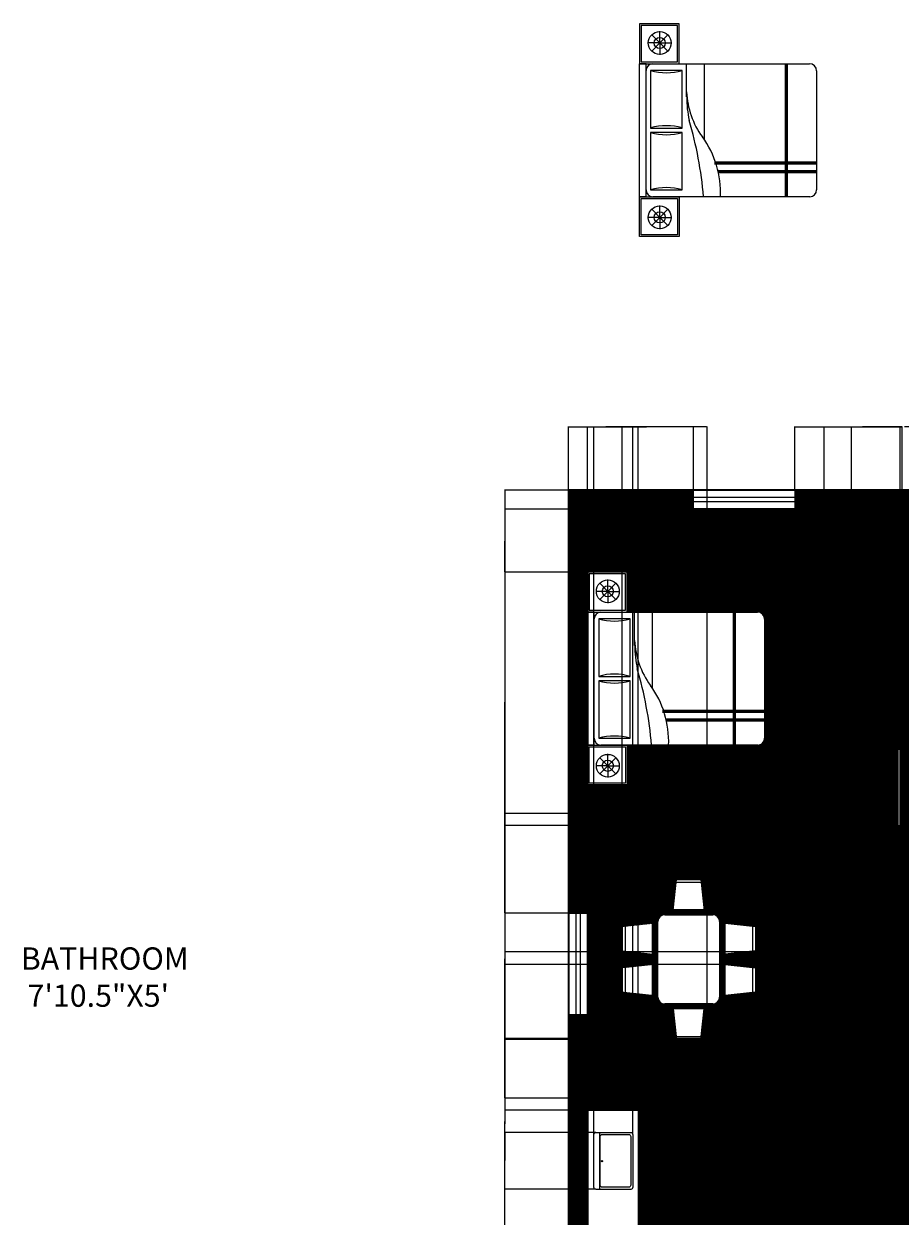
# Model space of a CAD drawing. Units: inches. Extents: x 205 to 1667, y -23 to 828.
# Tile 6 of 10: x 205 to 619, y 264 to 828. Entities that reach past the tile are written whole.
import ezdxf

# ---------------------------------------------------------------- set-up
doc = ezdxf.new("R2010")
doc.units = ezdxf.units.IN
doc.header["$MEASUREMENT"] = 0
for name, color, linetype, lineweight in [('A-ANNO-DIMS', 2, 'Continuous', 18), ('A-AREA-IDEN', 7, 'Continuous', 25), ('A-DOOR', 4, 'Continuous', 25), ('A-FLOR-CASE', 32, 'Continuous', 25), ('A-FLOR-FIXT', 9, 'Continuous', 18), ('A-FURN', 8, 'Continuous', 18), ('A-GLAZ', 4, 'Continuous', 18), ('A-WALL', 7, 'Continuous', 35)]:
    doc.layers.add(name, color=color, linetype=linetype, lineweight=lineweight)
doc.layers.add('A-FLOR-PATT', color=9, linetype='Continuous', lineweight=9, true_color=0xc7c8ca)
doc.styles.get("Standard").update_dxf_attribs({"font": 'arial.ttf'})
doc.dimstyles.get("Standard").update_dxf_attribs({"dimtxt": 0.18, "dimasz": 0.18, "dimexe": 0.18, "dimexo": 0.0625, "dimgap": 0.09, "dimtad": 0, "dimtih": 1, "dimtoh": 1, "dimdec": 4, "dimzin": 0, "dimdsep": 46, "dimtxsty": 'Standard', "dimcen": 0.09, "dimadec": 0, "dimazin": 0, "dimtfac": 1, "dimtdec": 4, "dimtofl": 0, "dimtmove": 0, "dimatfit": 3, "dimfxl": 1, "dimtolj": 1, "dimtzin": 0, "dimarcsym": 0})

# ---------------------------------------------------------------- blocks, each defined once
blk = doc.blocks.new('A$C068671E6')
for p, q in [((0, 1.55), (0, 2)), ((0, 2), (0.45, 2)), ((0.02, 1.57), (0.02, 1.98)), ((0.02, 1.98), (0.43, 1.98)), ((0.216, 1.77), (0.216, 1.905)), ((0.43, 1.98), (0.43, 1.57)), ((0.45, 2), (0.45, 1.55)), ((1.951, 2), (1.951, 1.55)), ((2.401, 2), (1.951, 2)), ((1.971, 1.98), (1.971, 1.57)), ((2.381, 1.98), (1.971, 1.98)), ((2.185, 1.77), (2.185, 1.905)), ((2.381, 1.57), (2.381, 1.98)), ((2.401, 1.55), (2.401, 2)), ((0.216, 1.77), (0.082, 1.77)), ((0.216, 1.77), (0.121, 1.865)), ((0.216, 1.77), (0.121, 1.675)), ((0.216, 1.77), (0.311, 1.865)), ((0.216, 1.77), (0.216, 1.636)), ((0.216, 1.77), (0.311, 1.675)), ((0.216, 1.77), (0.35, 1.77)), ((2.185, 1.77), (2.05, 1.77)), ((2.185, 1.77), (2.09, 1.865)), ((2.185, 1.77), (2.09, 1.675)), ((2.185, 1.77), (2.28, 1.865)), ((2.185, 1.77), (2.185, 1.636)), ((2.185, 1.77), (2.319, 1.77)), ((2.185, 1.77), (2.28, 1.675)), ((0.45, 1.55), (0, 1.55)), ((0.43, 1.57), (0.02, 1.57)), ((1.951, 1.55), (2.401, 1.55)), ((1.971, 1.57), (2.381, 1.57)), ((0.722, 1.115), (0.722, 0)), ((0.734, 1.115), (0.734, 0)), ((0.746, 1.115), (0.746, 0)), ((0.82, 1.151), (0.82, 0)), ((0.832, 1.151), (0.832, 0)), ((0.844, 1.151), (0.844, 0)), ((0.46, 0.352), (1.944, 0.352)), ((0.46, 0.34), (1.944, 0.34)), ((0.46, 0.328), (1.944, 0.328))]:
    blk.add_line(p, q)
at = {"linetype": 'ByBlock'}
for p, q in [((0.45, 1.924), (0.45, 2)), ((0.45, 2), (1.951, 2)), ((0.45, 1.924), (1.951, 1.924)), ((1.951, 1.924), (1.951, 2)), ((0.45, 0.076), (0.45, 1.848)), ((1.174, 1.873), (0.526, 1.873)), ((0.526, 1.873), (0.526, 1.518)), ((1.174, 1.518), (1.174, 1.873)), ((1.874, 1.873), (1.225, 1.873)), ((1.225, 1.873), (1.225, 1.518)), ((1.874, 1.518), (1.874, 1.873)), ((1.951, 1.848), (1.951, 0.08)), ((0.526, 1.518), (1.174, 1.518)), ((1.225, 1.518), (1.874, 1.518)), ((1.575, 1.467), (1.951, 1.467)), ((1.098, 1.264), (1.951, 1.264)), ((1.871, 0), (0.526, 0))]:
    blk.add_line(p, q, dxfattribs=at)
for centre, radius in [((0.216, 1.77), 0.129), ((2.185, 1.77), 0.129), ((0.216, 1.77), 0.0628), ((2.185, 1.77), 0.0628)]:
    blk.add_circle(centre, radius)
for centre, radius, start, end in [((0.526, 1.848), 0.0762, 90, 180), ((1.874, 1.848), 0.0762, 0, 90), ((-0.083, 1.695), 0.635, 343.7398, 16.2602), ((1.784, 1.695), 0.635, 163.7398, 196.2602), ((0.616, 1.695), 0.635, 343.7398, 16.2602), ((2.484, 1.695), 0.635, 163.7398, 196.2602), ((0.069, 5.66), 4.401, 274.9624, 286.3911), ((1.673, 0.534), 0.934, 92.5398, 126.0403), ((1.574, 0.247), 1.219, 89.9814, 102.4667), ((0.493, 2.153), 1.07, 267.6917, 306.1059), ((0.526, 0.076), 0.0762, 180, 270), ((1.871, 0.08), 0.08, 270, 0)]:
    blk.add_arc(centre, radius, start, end, dxfattribs=at)
blk = doc.blocks.new('A$C6D1B16CF')
for p, q in [((0.641, 1.5), (0.689, 1.943)), ((0.689, 1.943), (1.043, 1.943)), ((1.043, 1.943), (1.091, 1.5)), ((1.241, 1.5), (1.289, 1.943)), ((1.289, 1.943), (1.643, 1.943)), ((1.643, 1.943), (1.691, 1.5)), ((0.684, 1.9), (1.048, 1.9)), ((1.284, 1.9), (1.648, 1.9)), ((0.616, 1.421), (1.716, 1.421)), ((1.091, 1.5), (0.641, 1.5)), ((1.691, 1.5), (1.241, 1.5)), ((0.516, 0.621), (0.516, 1.321)), ((1.816, 1.321), (1.816, 0.621)), ((0, 1.146), (0.443, 1.194)), ((0, 0.792), (0, 1.146)), ((0.043, 0.787), (0.043, 1.151)), ((0.443, 1.194), (0.443, 0.744)), ((2.332, 1.146), (1.889, 1.194)), ((1.889, 1.194), (1.889, 0.744)), ((2.289, 0.787), (2.289, 1.151)), ((2.332, 0.792), (2.332, 1.146)), ((0.443, 0.744), (0, 0.792)), ((1.889, 0.744), (2.332, 0.792)), ((1.716, 0.521), (0.616, 0.521)), ((1.091, 0.443), (0.641, 0.443)), ((0.641, 0.443), (0.689, 0)), ((1.043, 0), (1.091, 0.443)), ((1.691, 0.443), (1.241, 0.443)), ((1.241, 0.443), (1.289, 0)), ((1.643, 0), (1.691, 0.443)), ((0.684, 0.043), (1.048, 0.043)), ((0.689, 0), (1.043, 0)), ((1.284, 0.043), (1.648, 0.043)), ((1.289, 0), (1.643, 0))]:
    blk.add_line(p, q)
for centre, start, end in [((0.616, 1.321), 90, 180), ((1.716, 1.321), 0, 90), ((0.616, 0.621), 180, 270), ((1.716, 0.621), 270, 0)]:
    blk.add_arc(centre, 0.1, start, end)
blk = doc.blocks.new('WIN-48IN')
for p, q in [((0, 0), (0, 9)), ((0, 9), (48, 9)), ((48, 9), (48, 0)), ((48, 5.5), (0, 5.5)), ((48, 3.5), (0, 3.5)), ((48, 0), (0, 0))]:
    blk.add_line(p, q)
blk = doc.blocks.new('DOOR-SINGLE-36IN')
for p, q in [((35, 0), (35, 36)), ((36, 0), (36, 36)), ((35, 0), (36, 0))]:
    blk.add_line(p, q)
blk.add_arc((35.5, 0.5), 35.5, 89.1931, 180.8069)
blk = doc.blocks.new('*D28')
at = {"layer": 'A-ANNO-DIMS', "color": 0, "lineweight": -2, "transparency": 16777216}
for p, q in [((583.31, 448.9), (583.31, 443.36)), ((619.44, 448.9), (619.44, 443.36)), ((583.49, 443.54), (600.01, 443.54)), ((619.26, 443.54), (602.73, 443.54))]:
    blk.add_line(p, q, dxfattribs=at)
at = {"layer": 'A-ANNO-DIMS', "color": 0, "transparency": 16777216}
for points in [[(583.49, 443.57), (583.49, 443.51), (583.31, 443.54)], [(619.26, 443.57), (619.26, 443.51), (619.44, 443.54)]]:
    blk.add_solid(points, dxfattribs=at)
at = {"layer": 'Defpoints', "color": 0, "transparency": 16777216}
for p in [(583.31, 448.96), (619.44, 448.96), (619.44, 443.54)]:
    blk.add_point(p, dxfattribs=at)
at = {"layer": 'A-ANNO-DIMS', "color": 0, "transparency": 16777216, "insert": (601.37, 443.54), "char_height": 0.18, "attachment_point": 5}
blk.add_mtext('\\A1;ROOM DOOR 36 TYP.', dxfattribs=at)
blk = doc.blocks.new('*D36')
at = {"layer": 'A-ANNO-DIMS', "color": 0, "lineweight": -2, "transparency": 16777216}
for p, q in [((487.8, 423.51), (476.32, 423.51)), ((476.5, 423.33), (476.5, 385.83)), ((476.5, 347.97), (476.5, 385.47)), ((487.8, 347.79), (476.32, 347.79))]:
    blk.add_line(p, q, dxfattribs=at)
at = {"layer": 'A-ANNO-DIMS', "color": 0, "transparency": 16777216}
for points in [[(476.47, 423.33), (476.53, 423.33), (476.5, 423.51)], [(476.47, 347.97), (476.53, 347.97), (476.5, 347.79)]]:
    blk.add_solid(points, dxfattribs=at)
at = {"layer": 'Defpoints', "color": 0, "transparency": 16777216}
for p in [(487.86, 423.51), (476.5, 347.79), (487.86, 347.79)]:
    blk.add_point(p, dxfattribs=at)
at = {"layer": 'A-ANNO-DIMS', "color": 0, "transparency": 16777216, "insert": (476.5, 385.65), "char_height": 0.18, "attachment_point": 5}
blk.add_mtext('\\A1;DINING SET 76', dxfattribs=at)
blk = doc.blocks.new('*D37')
at = {"layer": 'A-ANNO-DIMS', "color": 0, "lineweight": -2, "transparency": 16777216}
for p, q in [((487.86, 347.72), (487.86, 336.25)), ((550.95, 347.72), (550.95, 336.25)), ((488.04, 336.43), (519.19, 336.43)), ((550.77, 336.43), (519.63, 336.43))]:
    blk.add_line(p, q, dxfattribs=at)
at = {"layer": 'A-ANNO-DIMS', "color": 0, "transparency": 16777216}
for points in [[(488.04, 336.46), (488.04, 336.4), (487.86, 336.43)], [(550.77, 336.46), (550.77, 336.4), (550.95, 336.43)]]:
    blk.add_solid(points, dxfattribs=at)
at = {"layer": 'Defpoints', "color": 0, "transparency": 16777216}
for p in [(487.86, 347.79), (550.95, 347.79), (550.95, 336.43)]:
    blk.add_point(p, dxfattribs=at)
at = {"layer": 'A-ANNO-DIMS', "color": 0, "transparency": 16777216, "insert": (519.41, 336.43), "char_height": 0.18, "attachment_point": 5}
blk.add_mtext('\\A1;63', dxfattribs=at)
blk = doc.blocks.new('*D43')
at = {"layer": 'A-ANNO-DIMS', "color": 0, "lineweight": -2, "transparency": 16777216}
for p, q in [((462.37, 607.65), (432.19, 607.65)), ((432.37, 607.47), (432.37, 307.83)), ((432.37, 7.83), (432.37, 307.47)), ((462.37, 7.65), (432.19, 7.65))]:
    blk.add_line(p, q, dxfattribs=at)
at = {"layer": 'A-ANNO-DIMS', "color": 0, "transparency": 16777216}
for points in [[(432.34, 607.47), (432.4, 607.47), (432.37, 607.65)], [(432.34, 7.83), (432.4, 7.83), (432.37, 7.65)]]:
    blk.add_solid(points, dxfattribs=at)
at = {"layer": 'Defpoints', "color": 0, "transparency": 16777216}
for p in [(432.37, 607.65), (462.43, 607.65), (462.43, 7.65)]:
    blk.add_point(p, dxfattribs=at)
at = {"layer": 'A-ANNO-DIMS', "color": 0, "transparency": 16777216, "insert": (432.37, 307.65), "char_height": 0.18, "attachment_point": 5}
blk.add_mtext('\\A1;600', dxfattribs=at)
blk = doc.blocks.new('*D46')
at = {"layer": 'A-ANNO-DIMS', "color": 0, "lineweight": -2, "transparency": 16777216}
for p, q in [((462.43, 607.71), (462.43, 637.89)), ((462.61, 637.71), (491.61, 637.71)), ((521.39, 637.71), (492.39, 637.71)), ((521.57, 607.71), (521.57, 637.89))]:
    blk.add_line(p, q, dxfattribs=at)
at = {"layer": 'A-ANNO-DIMS', "color": 0, "transparency": 16777216}
for points in [[(462.61, 637.74), (462.61, 637.68), (462.43, 637.71)], [(521.39, 637.74), (521.39, 637.68), (521.57, 637.71)]]:
    blk.add_solid(points, dxfattribs=at)
at = {"layer": 'Defpoints', "color": 0, "transparency": 16777216}
for p in [(521.57, 637.71), (462.43, 607.65), (521.57, 607.65)]:
    blk.add_point(p, dxfattribs=at)
at = {"layer": 'A-ANNO-DIMS', "color": 0, "transparency": 16777216, "insert": (492, 637.71), "char_height": 0.18, "attachment_point": 5}
blk.add_mtext('\\A1;59.14', dxfattribs=at)
blk = doc.blocks.new('*D47')
at = {"layer": 'A-ANNO-DIMS', "color": 0, "lineweight": -2, "transparency": 16777216}
for p, q in [((569.57, 607.71), (569.57, 637.89)), ((569.75, 637.71), (620.6, 637.71)), ((672.35, 637.71), (621.51, 637.71)), ((672.53, 607.71), (672.53, 637.89))]:
    blk.add_line(p, q, dxfattribs=at)
at = {"layer": 'A-ANNO-DIMS', "color": 0, "transparency": 16777216}
for points in [[(569.75, 637.74), (569.75, 637.68), (569.57, 637.71)], [(672.35, 637.74), (672.35, 637.68), (672.53, 637.71)]]:
    blk.add_solid(points, dxfattribs=at)
at = {"layer": 'Defpoints', "color": 0, "transparency": 16777216}
for p in [(672.53, 637.71), (569.57, 607.65), (672.53, 607.65)]:
    blk.add_point(p, dxfattribs=at)
at = {"layer": 'A-ANNO-DIMS', "color": 0, "transparency": 16777216, "insert": (621.05, 637.71), "char_height": 0.18, "attachment_point": 5}
blk.add_mtext('\\A1;102.96', dxfattribs=at)
blk = doc.blocks.new('*D48')
at = {"layer": 'A-ANNO-DIMS', "color": 0, "lineweight": -2, "transparency": 16777216}
for p, q in [((462.37, 607.65), (432.19, 607.65)), ((432.37, 607.47), (432.37, 507.72)), ((432.37, 407.61), (432.37, 507.36)), ((462.37, 407.43), (432.19, 407.43))]:
    blk.add_line(p, q, dxfattribs=at)
at = {"layer": 'A-ANNO-DIMS', "color": 0, "transparency": 16777216}
for points in [[(432.34, 607.47), (432.4, 607.47), (432.37, 607.65)], [(432.34, 407.61), (432.4, 407.61), (432.37, 407.43)]]:
    blk.add_solid(points, dxfattribs=at)
at = {"layer": 'Defpoints', "color": 0, "transparency": 16777216}
for p in [(462.43, 607.65), (432.37, 407.43), (462.43, 407.43)]:
    blk.add_point(p, dxfattribs=at)
at = {"layer": 'A-ANNO-DIMS', "color": 0, "transparency": 16777216, "insert": (432.37, 507.54), "char_height": 0.18, "attachment_point": 5}
blk.add_mtext('\\A1;200.22', dxfattribs=at)
blk = doc.blocks.new('*D53')
at = {"layer": 'A-ANNO-DIMS', "color": 0, "lineweight": -2, "transparency": 16777216}
for p, q in [((471.43, 314.38), (471.43, 637.89)), ((471.61, 637.71), (483.21, 637.71)), ((495.25, 637.71), (483.65, 637.71)), ((495.43, 314.38), (495.43, 637.89))]:
    blk.add_line(p, q, dxfattribs=at)
at = {"layer": 'A-ANNO-DIMS', "color": 0, "transparency": 16777216}
for points in [[(471.61, 637.74), (471.61, 637.68), (471.43, 637.71)], [(495.25, 637.74), (495.25, 637.68), (495.43, 637.71)]]:
    blk.add_solid(points, dxfattribs=at)
at = {"layer": 'Defpoints', "color": 0, "transparency": 16777216}
for p in [(495.43, 637.71), (471.43, 314.32), (495.43, 314.32)]:
    blk.add_point(p, dxfattribs=at)
at = {"layer": 'A-ANNO-DIMS', "color": 0, "transparency": 16777216, "insert": (483.43, 637.71), "char_height": 0.18, "attachment_point": 5}
blk.add_mtext('\\A1;24', dxfattribs=at)
blk = doc.blocks.new('*D59')
at = {"layer": 'A-ANNO-DIMS', "color": 0, "lineweight": -2, "transparency": 16777216}
for p, q in [((666.24, 348.25), (432.19, 348.25)), ((432.37, 348.07), (432.37, 334.28)), ((432.37, 320.12), (432.37, 333.91)), ((666.24, 319.94), (432.19, 319.94))]:
    blk.add_line(p, q, dxfattribs=at)
at = {"layer": 'A-ANNO-DIMS', "color": 0, "transparency": 16777216}
for points in [[(432.34, 348.07), (432.4, 348.07), (432.37, 348.25)], [(432.34, 320.12), (432.4, 320.12), (432.37, 319.94)]]:
    blk.add_solid(points, dxfattribs=at)
at = {"layer": 'Defpoints', "color": 0, "transparency": 16777216}
for p in [(432.37, 348.25), (666.3, 348.25), (666.3, 319.94)]:
    blk.add_point(p, dxfattribs=at)
at = {"layer": 'A-ANNO-DIMS', "color": 0, "transparency": 16777216, "insert": (432.37, 334.09), "char_height": 0.18, "attachment_point": 5}
blk.add_mtext('\\A1;28.31', dxfattribs=at)
blk = doc.blocks.new('*D60')
at = {"layer": 'A-ANNO-DIMS', "color": 0, "lineweight": -2, "transparency": 16777216}
for p, q in [((672.24, 389.16), (432.19, 389.16)), ((432.37, 388.98), (432.37, 386.33)), ((432.37, 383.31), (432.37, 385.96)), ((672.24, 383.13), (432.19, 383.13))]:
    blk.add_line(p, q, dxfattribs=at)
at = {"layer": 'A-ANNO-DIMS', "color": 0, "transparency": 16777216}
for points in [[(432.34, 388.98), (432.4, 388.98), (432.37, 389.16)], [(432.34, 383.31), (432.4, 383.31), (432.37, 383.13)]]:
    blk.add_solid(points, dxfattribs=at)
at = {"layer": 'Defpoints', "color": 0, "transparency": 16777216}
for p in [(672.3, 389.16), (432.37, 383.13), (672.3, 383.13)]:
    blk.add_point(p, dxfattribs=at)
at = {"layer": 'A-ANNO-DIMS', "color": 0, "transparency": 16777216, "insert": (432.37, 386.14), "char_height": 0.18, "attachment_point": 5}
blk.add_mtext('\\A1;6.026', dxfattribs=at)
blk = doc.blocks.new('*D64')
at = {"layer": 'A-ANNO-DIMS', "color": 0, "lineweight": -2, "transparency": 16777216}
for p, q in [((471.43, 454.59), (471.43, -22.59)), ((583.44, 454.59), (583.44, -22.59)), ((471.61, -22.41), (527.16, -22.41)), ((583.26, -22.41), (527.71, -22.41))]:
    blk.add_line(p, q, dxfattribs=at)
at = {"layer": 'A-ANNO-DIMS', "color": 0, "transparency": 16777216}
for points in [[(471.61, -22.38), (471.61, -22.44), (471.43, -22.41)], [(583.26, -22.38), (583.26, -22.44), (583.44, -22.41)]]:
    blk.add_solid(points, dxfattribs=at)
at = {"layer": 'Defpoints', "color": 0, "transparency": 16777216}
for p in [(471.43, 454.65), (583.44, 454.65), (583.44, -22.41)]:
    blk.add_point(p, dxfattribs=at)
at = {"layer": 'A-ANNO-DIMS', "color": 0, "transparency": 16777216, "insert": (527.44, -22.41), "char_height": 0.18, "attachment_point": 5}
blk.add_mtext('\\A1;112', dxfattribs=at)
blk = doc.blocks.new('*D72')
at = {"layer": 'A-ANNO-DIMS', "color": 0, "lineweight": -2, "transparency": 16777216}
for p, q in [((471.37, 598.65), (432.19, 598.65)), ((432.37, 598.47), (432.37, 583.93)), ((432.37, 569.02), (432.37, 583.57)), ((471.37, 568.84), (432.19, 568.84))]:
    blk.add_line(p, q, dxfattribs=at)
at = {"layer": 'A-ANNO-DIMS', "color": 0, "transparency": 16777216}
for points in [[(432.34, 598.47), (432.4, 598.47), (432.37, 598.65)], [(432.34, 569.02), (432.4, 569.02), (432.37, 568.84)]]:
    blk.add_solid(points, dxfattribs=at)
at = {"layer": 'Defpoints', "color": 0, "transparency": 16777216}
for p in [(471.43, 598.65), (432.37, 568.84), (471.43, 568.84)]:
    blk.add_point(p, dxfattribs=at)
at = {"layer": 'A-ANNO-DIMS', "color": 0, "transparency": 16777216, "insert": (432.37, 583.75), "char_height": 0.18, "attachment_point": 5}
blk.add_mtext('\\A1;29.807', dxfattribs=at)
blk = doc.blocks.new('*D74')
at = {"layer": 'A-ANNO-DIMS', "color": 0, "lineweight": -2, "transparency": 16777216}
for p, q in [((471.43, 407.49), (471.43, 637.89)), ((471.61, 637.71), (479.19, 637.71)), ((487.68, 637.71), (480.1, 637.71)), ((487.86, 401.21), (487.86, 637.89))]:
    blk.add_line(p, q, dxfattribs=at)
at = {"layer": 'A-ANNO-DIMS', "color": 0, "transparency": 16777216}
for points in [[(471.61, 637.74), (471.61, 637.68), (471.43, 637.71)], [(487.68, 637.74), (487.68, 637.68), (487.86, 637.71)]]:
    blk.add_solid(points, dxfattribs=at)
at = {"layer": 'Defpoints', "color": 0, "transparency": 16777216}
for p in [(487.86, 637.71), (471.43, 407.43), (487.86, 401.15)]:
    blk.add_point(p, dxfattribs=at)
at = {"layer": 'A-ANNO-DIMS', "color": 0, "transparency": 16777216, "insert": (479.65, 637.71), "char_height": 0.18, "attachment_point": 5}
blk.add_mtext('\\A1;16.432', dxfattribs=at)
blk = doc.blocks.new('*D75')
at = {"layer": 'A-ANNO-DIMS', "color": 0, "lineweight": -2, "transparency": 16777216}
for p, q in [((513.5, 347.79), (432.19, 347.79)), ((432.37, 347.61), (432.37, 334.04)), ((432.37, 320.12), (432.37, 333.68)), ((471.37, 319.94), (432.19, 319.94))]:
    blk.add_line(p, q, dxfattribs=at)
at = {"layer": 'A-ANNO-DIMS', "color": 0, "transparency": 16777216}
for points in [[(432.34, 347.61), (432.4, 347.61), (432.37, 347.79)], [(432.34, 320.12), (432.4, 320.12), (432.37, 319.94)]]:
    blk.add_solid(points, dxfattribs=at)
at = {"layer": 'Defpoints', "color": 0, "transparency": 16777216}
for p in [(432.37, 347.79), (513.57, 347.79), (471.43, 319.94)]:
    blk.add_point(p, dxfattribs=at)
at = {"layer": 'A-ANNO-DIMS', "color": 0, "transparency": 16777216, "insert": (432.37, 333.86), "char_height": 0.18, "attachment_point": 5}
blk.add_mtext('\\A1;27.85', dxfattribs=at)
blk = doc.blocks.new('*D76')
at = {"layer": 'A-ANNO-DIMS', "color": 0, "lineweight": -2, "transparency": 16777216}
for p, q in [((471.43, 213.99), (471.43, 637.89)), ((471.61, 637.71), (499.41, 637.71)), ((527.85, 637.71), (500.05, 637.71)), ((528.03, 216.24), (528.03, 637.89))]:
    blk.add_line(p, q, dxfattribs=at)
at = {"layer": 'A-ANNO-DIMS', "color": 0, "transparency": 16777216}
for points in [[(471.61, 637.74), (471.61, 637.68), (471.43, 637.71)], [(527.85, 637.74), (527.85, 637.68), (528.03, 637.71)]]:
    blk.add_solid(points, dxfattribs=at)
at = {"layer": 'Defpoints', "color": 0, "transparency": 16777216}
for p in [(528.03, 637.71), (528.03, 216.18), (471.43, 213.93)]:
    blk.add_point(p, dxfattribs=at)
at = {"layer": 'A-ANNO-DIMS', "color": 0, "transparency": 16777216, "insert": (499.73, 637.71), "char_height": 0.18, "attachment_point": 5}
blk.add_mtext('\\A1;56.6', dxfattribs=at)
blk = doc.blocks.new('*D77')
at = {"layer": 'A-ANNO-DIMS', "color": 0, "lineweight": -2, "transparency": 16777216}
for p, q in [((471.37, 314.32), (432.19, 314.32)), ((432.37, 314.14), (432.37, 309.22)), ((432.37, 303.94), (432.37, 308.86)), ((475.44, 303.76), (432.19, 303.76))]:
    blk.add_line(p, q, dxfattribs=at)
at = {"layer": 'A-ANNO-DIMS', "color": 0, "transparency": 16777216}
for points in [[(432.34, 314.14), (432.4, 314.14), (432.37, 314.32)], [(432.34, 303.94), (432.4, 303.94), (432.37, 303.76)]]:
    blk.add_solid(points, dxfattribs=at)
at = {"layer": 'Defpoints', "color": 0, "transparency": 16777216}
for p in [(471.43, 314.32), (432.37, 303.76), (475.5, 303.76)]:
    blk.add_point(p, dxfattribs=at)
at = {"layer": 'A-ANNO-DIMS', "color": 0, "transparency": 16777216, "insert": (432.37, 309.04), "char_height": 0.18, "attachment_point": 5}
blk.add_mtext('\\A1;10.562', dxfattribs=at)
blk = doc.blocks.new('*D78')
at = {"layer": 'A-ANNO-DIMS', "color": 0, "lineweight": -2, "transparency": 16777216}
for p, q in [((474.5, 302.82), (474.5, 637.89)), ((474.68, 637.71), (483.25, 637.71)), ((492.73, 637.71), (484.16, 637.71)), ((492.91, 302.82), (492.91, 637.89))]:
    blk.add_line(p, q, dxfattribs=at)
at = {"layer": 'A-ANNO-DIMS', "color": 0, "transparency": 16777216}
for points in [[(474.68, 637.74), (474.68, 637.68), (474.5, 637.71)], [(492.73, 637.74), (492.73, 637.68), (492.91, 637.71)]]:
    blk.add_solid(points, dxfattribs=at)
at = {"layer": 'Defpoints', "color": 0, "transparency": 16777216}
for p in [(492.91, 637.71), (474.5, 302.76), (492.91, 302.76)]:
    blk.add_point(p, dxfattribs=at)
at = {"layer": 'A-ANNO-DIMS', "color": 0, "transparency": 16777216, "insert": (483.7, 637.71), "char_height": 0.18, "attachment_point": 5}
blk.add_mtext('\\A1;18.413', dxfattribs=at)
blk = doc.blocks.new('*D79')
at = {"layer": 'A-ANNO-DIMS', "color": 0, "lineweight": -2, "transparency": 16777216}
for p, q in [((475.44, 303.76), (432.19, 303.76)), ((432.37, 303.58), (432.37, 290.46)), ((432.37, 276.99), (432.37, 290.1)), ((475.44, 276.81), (432.19, 276.81))]:
    blk.add_line(p, q, dxfattribs=at)
at = {"layer": 'A-ANNO-DIMS', "color": 0, "transparency": 16777216}
for points in [[(432.34, 303.58), (432.4, 303.58), (432.37, 303.76)], [(432.34, 276.99), (432.4, 276.99), (432.37, 276.81)]]:
    blk.add_solid(points, dxfattribs=at)
at = {"layer": 'Defpoints', "color": 0, "transparency": 16777216}
for p in [(475.5, 303.76), (432.37, 276.81), (475.5, 276.81)]:
    blk.add_point(p, dxfattribs=at)
at = {"layer": 'A-ANNO-DIMS', "color": 0, "transparency": 16777216, "insert": (432.37, 290.28), "char_height": 0.18, "attachment_point": 5}
blk.add_mtext('\\A1;26.95', dxfattribs=at)
blk = doc.blocks.new('*D80')
at = {"layer": 'A-ANNO-DIMS', "color": 0, "lineweight": -2, "transparency": 16777216}
for p, q in [((596.44, 213.99), (596.44, 637.89)), ((596.62, 637.71), (608.22, 637.71)), ((620.26, 637.71), (608.66, 637.71)), ((620.44, 213.99), (620.44, 637.89))]:
    blk.add_line(p, q, dxfattribs=at)
at = {"layer": 'A-ANNO-DIMS', "color": 0, "transparency": 16777216}
for points in [[(596.62, 637.74), (596.62, 637.68), (596.44, 637.71)], [(620.26, 637.74), (620.26, 637.68), (620.44, 637.71)]]:
    blk.add_solid(points, dxfattribs=at)
at = {"layer": 'Defpoints', "color": 0, "transparency": 16777216}
for p in [(596.44, 637.71), (596.44, 213.93), (620.44, 213.93)]:
    blk.add_point(p, dxfattribs=at)
at = {"layer": 'A-ANNO-DIMS', "color": 0, "transparency": 16777216, "insert": (608.44, 637.71), "char_height": 0.18, "attachment_point": 5}
blk.add_mtext('\\A1;24', dxfattribs=at)
blk = doc.blocks.new('*D85')
at = {"layer": 'A-ANNO-DIMS', "color": 0, "lineweight": -2, "transparency": 16777216}
for p, q in [((471.37, 448.96), (432.19, 448.96)), ((432.37, 448.78), (432.37, 384.63)), ((432.37, 320.12), (432.37, 384.27)), ((471.37, 319.94), (432.19, 319.94))]:
    blk.add_line(p, q, dxfattribs=at)
at = {"layer": 'A-ANNO-DIMS', "color": 0, "transparency": 16777216}
for points in [[(432.34, 448.78), (432.4, 448.78), (432.37, 448.96)], [(432.34, 320.12), (432.4, 320.12), (432.37, 319.94)]]:
    blk.add_solid(points, dxfattribs=at)
at = {"layer": 'Defpoints', "color": 0, "transparency": 16777216}
for p in [(471.43, 448.96), (432.37, 319.94), (471.43, 319.94)]:
    blk.add_point(p, dxfattribs=at)
at = {"layer": 'A-ANNO-DIMS', "color": 0, "transparency": 16777216, "insert": (432.37, 384.45), "char_height": 0.18, "attachment_point": 5}
blk.add_mtext('\\A1;129.02', dxfattribs=at)
blk = doc.blocks.new('*D86')
at = {"layer": 'A-ANNO-DIMS', "color": 0, "lineweight": -2, "transparency": 16777216}
for p, q in [((583.44, 320), (583.44, 637.89)), ((583.62, 637.71), (601.22, 637.71)), ((619.26, 637.71), (601.66, 637.71)), ((619.44, 320), (619.44, 637.89))]:
    blk.add_line(p, q, dxfattribs=at)
at = {"layer": 'A-ANNO-DIMS', "color": 0, "transparency": 16777216}
for points in [[(583.62, 637.74), (583.62, 637.68), (583.44, 637.71)], [(619.26, 637.74), (619.26, 637.68), (619.44, 637.71)]]:
    blk.add_solid(points, dxfattribs=at)
at = {"layer": 'Defpoints', "color": 0, "transparency": 16777216}
for p in [(619.44, 637.71), (583.44, 319.94), (619.44, 319.94)]:
    blk.add_point(p, dxfattribs=at)
at = {"layer": 'A-ANNO-DIMS', "color": 0, "transparency": 16777216, "insert": (601.44, 637.71), "char_height": 0.18, "attachment_point": 5}
blk.add_mtext('\\A1;36', dxfattribs=at)
blk = doc.blocks.new('*D88')
at = {"layer": 'A-ANNO-DIMS', "color": 0, "lineweight": -2, "transparency": 16777216}
for p, q in [((471.37, 454.65), (432.19, 454.65)), ((432.37, 454.47), (432.37, 451.99)), ((432.37, 449.14), (432.37, 451.63)), ((471.37, 448.96), (432.19, 448.96))]:
    blk.add_line(p, q, dxfattribs=at)
at = {"layer": 'A-ANNO-DIMS', "color": 0, "transparency": 16777216}
for points in [[(432.34, 454.47), (432.4, 454.47), (432.37, 454.65)], [(432.34, 449.14), (432.4, 449.14), (432.37, 448.96)]]:
    blk.add_solid(points, dxfattribs=at)
at = {"layer": 'Defpoints', "color": 0, "transparency": 16777216}
for p in [(471.43, 454.65), (432.37, 448.96), (471.43, 448.96)]:
    blk.add_point(p, dxfattribs=at)
at = {"layer": 'A-ANNO-DIMS', "color": 0, "transparency": 16777216, "insert": (432.37, 451.81), "char_height": 0.18, "attachment_point": 5}
blk.add_mtext('\\A1;5.688', dxfattribs=at)

msp = doc.modelspace()

# ---------------------------------------------------------------- hatches: boundary and pattern name
at = {"layer": 'A-FLOR-PATT'}
h = msp.add_hatch(dxfattribs=at)
h.set_pattern_fill('ANSI31', color=256)
h.paths.add_polyline_path([(774.4305, 607.6511), (720.5338, 607.6511), (720.5338, 598.6511), (727.9933, 598.6511), (746.8614, 598.6511), (765.4305, 598.6511), (765.4305, 454.6511), (759.5298, 454.6511), (759.5298, 448.9635), (765.4305, 448.9635), (765.4305, 428.0602), (774.4305, 428.0602)])
h.paths.add_polyline_path([(765.4305, 598.6511), (746.8614, 598.6511), (746.8614, 579.7829), (727.9933, 579.7829), (727.9933, 518.1387, -0.41421701), (724.6389, 514.7843), (668.2693, 514.7843, -0.41421356), (665.0743, 517.9793), (665.0743, 579.7829), (646.2062, 579.7829), (646.2062, 598.6511), (626.3468, 598.6511), (626.3468, 454.6511), (628.3468, 454.6511), (628.3468, 484.9635, -0.41421356), (664.3468, 449.9635), (664.3468, 454.6511), (729.3305, 454.6511), (758.5298, 454.6511), (759.5298, 454.6511), (765.4305, 454.6511)])
h.paths.add_polyline_path([(621.4404, 598.6511), (471.4305, 598.6511), (471.4305, 568.8442), (490.2987, 568.8442), (490.2987, 549.9761), (551.9429, 549.9761, -0.41421701), (555.2973, 546.6217), (555.2973, 490.2521, -0.41421356), (552.1023, 487.0571), (490.2987, 487.0571), (490.2987, 468.189), (471.4305, 468.189), (471.4305, 454.6511), (583.4404, 454.6511), (583.4404, 449.9635, -0.41421356), (619.4404, 484.9635), (619.4404, 454.6511), (621.4404, 454.6511)])
h.paths.add_polyline_path([(672.5338, 607.6511), (569.5707, 607.6511), (569.5707, 598.6511), (621.4404, 598.6511), (621.4404, 454.6511), (619.4404, 454.6511), (619.4404, 448.9635), (628.3468, 448.9635), (628.3468, 454.6511), (626.3468, 454.6511), (626.3468, 598.6511), (646.2062, 598.6511), (665.0743, 598.6511), (672.5338, 598.6511)])
h.paths.add_polyline_path([(521.5707, 607.6511), (462.4305, 607.6511), (462.4305, 407.4306), (471.4305, 407.4306), (471.4305, 448.9635), (583.4404, 448.9635, -0.0070419), (583.4404, 449.9635), (583.4404, 454.6511), (471.4305, 454.6511), (471.4305, 468.189), (471.4305, 487.0571), (471.4305, 549.9761), (471.4305, 568.8442), (471.4305, 598.6511), (521.5707, 598.6511)])
h.paths.add_polyline_path([(471.4305, 314.3187), (583.4404, 314.3187), (583.4404, 319.9388), (471.4305, 319.9388), (471.4305, 359.4306), (462.4305, 359.4306), (462.4305, 7.6511), (471.4305, 7.6511), (471.4305, 204.9321), (521.9355, 204.9321), (521.9355, 213.9321), (471.4305, 213.9321)])
h.paths.add_polyline_path([(774.4305, 410.0602), (765.4305, 410.0602), (765.4305, 389.1569), (672.3024, 389.1569), (672.3024, 448.9635), (681.1739, 448.9635, -0.18532444), (681.6564, 449.1487), (698.6035, 449.1487), (729.3305, 448.9635), (729.3305, 454.6511), (664.3468, 454.6511), (664.3468, 449.9635, -0.0070419), (664.3468, 448.9635), (666.3024, 448.9635), (666.3024, 378.2485), (672.3024, 378.2485), (672.3024, 383.1306), (765.4305, 383.1306), (765.4305, 360.5347), (774.4305, 360.5347)])
h.paths.add_polyline_path([(774.4305, 342.5347), (765.4305, 342.5347), (765.4305, 319.9388), (672.3024, 319.9388), (672.3024, 348.5574), (671.0896, 348.5574, -0.04071533), (666.3024, 348.2485), (666.3024, 319.9388), (664.3468, 319.9388, -0.0070419), (664.3468, 318.9388), (664.3468, 314.3187), (765.4305, 314.3187), (765.4305, 290.8426), (774.4305, 290.8426)])
h.paths.add_polyline_path([(774.4305, 242.8426), (765.4305, 242.8426), (765.4305, 104.6382), (626.3468, 104.6382), (626.3468, 110.5917), (617.3468, 110.5917), (617.3468, 95.6382), (765.4305, 95.6382), (765.4305, 16.6511), (621.2232, 16.6511), (621.2232, 7.6511), (774.4305, 7.6511)])
h.paths.add_polyline_path([(626.3468, 314.3187), (628.3468, 314.3187), (628.3468, 319.9388), (619.4404, 319.9388), (619.4404, 314.3187), (620.4404, 314.3187), (620.4404, 213.9321), (569.9355, 213.9321), (569.9355, 204.9321), (617.3468, 204.9321), (617.3468, 153.3751), (626.3468, 153.3751)])
h.paths.add_polyline_path([(620.4404, 314.3187), (619.4404, 314.3187), (619.4404, 319.9388), (628.3468, 319.9388), (629.3468, 319.9388), (629.3468, 283.9388, 0.40598745), (664.3468, 318.9388), (664.3468, 319.9388), (666.3024, 319.9388), (666.3024, 348.2485), (666.3024, 377.2485), (666.3024, 378.2485), (666.3024, 448.9635), (664.3468, 448.9635), (664.3468, 449.9635, 0.40598745), (629.3468, 484.9635), (629.3468, 448.9635), (628.3468, 448.9635), (619.4404, 448.9635), (618.4404, 448.9635), (618.4404, 484.9635, 0.40598745), (583.4404, 449.9635), (583.4404, 448.9635), (471.4305, 448.9635), (471.4305, 407.4306), (471.4305, 359.4306), (471.4305, 319.9388), (583.4404, 319.9388), (583.4404, 314.3187), (495.4305, 314.3187), (495.4305, 237.9321), (620.4404, 237.9321)])
h.paths.add_polyline_path([(525.0876, 347.7863), (513.5657, 347.7863), (512.0216, 362.1672), (526.6317, 362.1672)], flags=16)
h.paths.add_polyline_path([(550.9499, 370.1471), (536.569, 368.6029), (536.569, 383.2131), (550.9499, 381.6689)], flags=16)
h.paths.add_polyline_path([(530.7713, 364.5431), (508.0415, 364.5431, -0.41421356), (504.7944, 367.7902), (504.7944, 403.5085, -0.41421356), (508.0415, 406.7556), (530.7713, 406.7556, -0.41421356), (534.0184, 403.5085), (534.0184, 367.7902, -0.41421356)], flags=16)
h.paths.add_polyline_path([(550.9499, 389.6298), (536.569, 388.0856), (536.569, 402.6958), (550.9499, 401.1516)], flags=16)
h.paths.add_polyline_path([(502.2439, 368.6029), (487.863, 370.1471), (487.863, 381.6689), (502.2439, 383.2131)], flags=16)
h.paths.add_polyline_path([(502.2439, 388.0856), (487.863, 389.6298), (487.863, 401.1516), (502.2439, 402.6958)], flags=16)
h.paths.add_polyline_path([(526.6317, 409.1315), (512.0216, 409.1315), (513.5657, 423.5124), (525.0876, 423.5124)], flags=16)
h.paths.add_polyline_path([(765.4305, 290.8426), (765.4305, 314.3187), (664.3468, 314.3187), (664.3468, 318.9388, -0.41421356), (628.3468, 283.9388), (628.3468, 314.3187), (626.3468, 314.3187), (626.3468, 153.3751), (638.3468, 153.3751, -0.4196361), (617.5748, 131.9834, -0.4196361), (638.3468, 110.5917), (626.3468, 110.5917), (626.3468, 104.6382), (765.4305, 104.6382), (765.4305, 242.8426)])
h.paths.add_polyline_path([(691.5064, 243.4363), (693.2483, 243.4363), (725.4984, 243.4363), (725.4984, 241.7329), (725.4984, 177.0512), (723.7564, 177.0512), (691.5064, 177.0512), (691.5064, 178.7545)], flags=16)
h.paths.add_polyline_path([(689.8658, 265.2977), (689.8658, 296.6873, -0.41421356), (690.8346, 297.6561), (724.6111, 297.6561, -0.41421356), (725.5799, 296.6873), (725.5799, 265.2977, -0.41421356), (724.6111, 264.3289), (690.8346, 264.3289, -0.41421356)], flags=16)
h.paths.add_polyline_path([(694.1286, 265.6852), (694.1286, 288.9368, -0.41421356), (695.0974, 289.9056), (720.3483, 289.9056, -0.41421356), (721.3171, 288.9368), (721.3171, 265.6852, -0.04533947), (721.3013, 265.5106, -0.3531705), (720.3282, 264.7164), (695.0974, 264.7164, -0.41421356)], flags=0)
h.paths.add_polyline_path([(694.1286, 291.2619), (694.1286, 294.7497, -0.41421356), (695.0974, 295.7185), (720.3483, 295.7185, -0.41421356), (721.3171, 294.7497), (721.3171, 291.2619, -0.41421356), (720.3483, 290.2931), (695.0974, 290.2931, -0.41421356)], flags=0)
h.paths.add_polyline_path([(734.4369, 244.6615, -0.41421356), (735.2682, 245.4928), (762.2019, 245.4928, -0.41421356), (763.0332, 244.6615), (763.0332, 168.183, -0.41421356), (762.2019, 167.3517), (735.2682, 167.3517, -0.41421356), (734.4369, 168.183)], flags=16)
h.paths.add_polyline_path([(761.7032, 242.1676), (761.7032, 170.6768), (735.6007, 171.0093, -0.41421356), (734.7694, 171.8406), (734.7694, 193.5102, -0.56972741), (735.6007, 194.674, -0.41421356), (734.7694, 195.5053), (734.7694, 217.3423, -0.56972741), (735.6007, 218.5061, -0.41421356), (734.7694, 219.3374), (734.7694, 241.0038, -0.41421356), (735.6007, 241.8351), (735.1643, 242.1676)], flags=16)
h.paths.add_polyline_path([(757.5467, 171.0093), (760.5393, 171.0093, 0.41421356), (761.3706, 171.8406), (761.3706, 193.5102, 0.41421356), (760.5393, 194.3415), (757.5467, 194.3415, 0.41421356), (756.7154, 193.5102), (756.7155, 171.8534, 0.41871477)], flags=0)
h.paths.add_polyline_path([(756.7154, 241.0038, -0.41421356), (757.5467, 241.8351), (760.5393, 241.8351, -0.41421356), (761.3706, 241.0038), (761.3706, 219.3374, -0.41421356), (760.5393, 218.5061), (760.5393, 218.1736, -0.41421356), (761.3706, 217.3423), (761.3706, 195.5053, -0.41421356), (760.5393, 194.674), (757.5467, 194.674, -0.56972741), (756.3829, 195.5053, -0.41421356), (755.5516, 194.674), (755.5516, 194.3415, -0.41421356), (756.3829, 193.5102), (756.7154, 171.8406), (756.3829, 193.5102, 0.41421356), (755.5516, 194.3415), (735.6007, 194.674), (755.5516, 194.674, 0.41421356), (756.3829, 195.5053), (756.3829, 217.3423, 0.41421356), (755.5516, 218.1736), (735.6007, 218.5061), (755.5516, 218.5061, 0.41421356), (756.3829, 219.3374)], flags=0)
h.paths.add_polyline_path([(694.5151, 150.3608), (728.2916, 150.3608, -0.41421356), (729.2604, 149.3919), (729.2604, 118.0023, -0.41421356), (728.2916, 117.0335), (694.5151, 117.0335, -0.41421356), (693.5463, 118.0023), (693.5463, 149.3919, -0.41421356)], flags=16)
h.paths.add_polyline_path([(724.0288, 149.9732, -0.41421356), (724.9977, 149.0044), (724.9977, 125.7529, -0.41421356), (724.0288, 124.784), (698.7779, 124.784, -0.41421356), (697.8091, 125.7529), (697.8091, 149.0044, -0.04533947), (697.825, 149.179, -0.3531705), (698.798, 149.9732)], flags=0)
h.paths.add_polyline_path([(698.7779, 124.3965), (724.0288, 124.3965, -0.41421356), (724.9977, 123.4277), (724.9977, 119.94, -0.41421356), (724.0288, 118.9711), (698.7779, 118.9711, -0.41421356), (697.8091, 119.94), (697.8091, 123.4277, -0.41421356)], flags=0)

# ---------------------------------------------------------------- linework, layer by layer
at = {"layer": 'A-FLOR-CASE'}
msp.add_line((495.4305, 314.3187), (495.4305, 237.9321), dxfattribs=at)
at = {"layer": 'A-FLOR-FIXT'}
msp.add_line((477.1954, 303.7567), (477.1954, 276.8058), dxfattribs=at)
for points in [[(475.4977, 303.7567), (491.9102, 303.7567, -0.41421356), (492.9102, 302.7567), (492.9102, 277.8058, -0.41421356), (491.9102, 276.8058), (475.4977, 276.8058, -0.41421356), (474.4977, 277.8058), (474.4977, 302.7567, -0.41421356)], [(477.4462, 278.8058), (477.4462, 301.7567, -0.41421356), (478.4462, 302.7567), (490.9102, 302.7567, -0.41421356), (491.9102, 301.7567), (491.9102, 278.8058, -0.41421356), (490.9102, 277.8058), (478.4462, 277.8058, -0.41421356)]]:
    msp.add_lwpolyline(points, format="xyb", close=True, dxfattribs=at)
msp.add_circle((478.2851, 290.1328), 0.3205, dxfattribs=at)
at = {"layer": 'A-WALL'}
for p, q in [((774.4305, 607.6511), (462.4305, 607.6511)), ((462.4305, 607.6511), (462.4305, 7.6511)), ((471.4305, 598.6511), (471.4305, 454.6511)), ((621.4404, 598.6511), (471.4305, 598.6511)), ((583.4404, 454.6511), (471.4305, 454.6511)), ((583.4404, 454.6511), (583.4404, 448.9635)), ((471.4305, 449.9635), (471.4305, 319.9388)), ((583.4404, 448.9635), (471.4305, 448.9635)), ((583.4404, 319.9388), (471.4305, 319.9388)), ((583.4404, 319.9388), (583.4404, 314.3187)), ((471.4305, 314.3187), (471.4305, 213.9321)), ((583.4404, 314.3187), (471.4305, 314.3187))]:
    msp.add_line(p, q, dxfattribs=at)

# ---------------------------------------------------------------- block references
at = {"layer": 'A-DOOR'}
msp.add_blockref('DOOR-SINGLE-36IN', (583.44, 448.964), dxfattribs=at)
at = {"layer": 'A-FURN'}
for name, p, xscale, yscale, zscale, rotation in [('A$C068671E6', (579.885, 727.7115), 41.92918703190525, 41.92918703190525, 41.92918703190525, 90), ('A$C068671E6', (555.2973, 468.189), 41.92918703190525, 41.92918703190525, 41.92918703190525, 90), ('A$C6D1B16CF', (487.863, 423.5124), 32.4711341177044, 32.4711341177044, 32.4711341177044, 270)]:
    msp.add_blockref(name, p, dxfattribs=dict(at, xscale=xscale, yscale=yscale, zscale=zscale, rotation=rotation))
at = {"layer": 'A-GLAZ'}
msp.add_blockref('WIN-48IN', (521.5709, 598.651), dxfattribs=at)
at = {"layer": 'A-GLAZ', "rotation": 89.99999999999991}
msp.add_blockref('WIN-48IN', (471.4306, 359.4308), dxfattribs=at)

# ---------------------------------------------------------------- texts
at = {"layer": 'A-AREA-IDEN', "attachment_point": 1}
for s, heights, insert, char_height in [('M BED ROOM\\P12\'6"X12\'', [44.9455], (524.5875, 586.4215), 10.53941), ('  DINING\\P16\'3"X10\'3"', [33.0594], (575.6629, 403.7792), 10.539409), ('BATHROOM\\P 7\'10.5"X5\'', [37.0032], (203.2664, 391.3085), 10.539409), ('KITCHEN\\P12\'6"X10\'', [48.204], (517.0093, 300.1661), 10.53941)]:
    msp.add_mtext_dynamic_manual_height_columns(s, width=126.149246, gutter_width=52.697, heights=heights, dxfattribs=dict(at, insert=insert, char_height=char_height))

# ---------------------------------------------------------------- dimensions: what is measured, and where the dimension line sits
at = {"layer": 'A-ANNO-DIMS'}
for base, p1, p2, override, picture, middle in [((521.5707, 637.7086), (462.4305, 607.6511), (521.5707, 607.6511), {"dimdec": 2, "dimlfac": 1, "dimrnd": 0, "dimzin": 0, "dimdsep": 46, "dimlunit": 2}, '*D46', (492.0006, 637.7086)), ((495.4305, 637.7086), (471.4305, 314.3187), (495.4305, 314.3187), {"dimdec": 0, "dimlfac": 1, "dimrnd": 0, "dimzin": 0, "dimdsep": 46, "dimlunit": 2}, '*D53', (483.4305, 637.7086)), ((487.86295, 637.70858), (471.43055, 407.43064), (487.86295, 401.15161), {"dimdec": 3, "dimlfac": 1, "dimrnd": 0, "dimzin": 0, "dimdsep": 46, "dimlunit": 2}, '*D74', (479.64675, 637.70858)), ((528.0312, 637.7086), (471.4305, 213.9321), (528.0312, 216.1782), {"dimdec": 1, "dimlfac": 1, "dimrnd": 0, "dimzin": 0, "dimdsep": 46, "dimlunit": 2}, '*D76', (499.7309, 637.7086)), ((492.91021, 637.70858), (474.4977, 302.75673), (492.91021, 302.75673), {"dimdec": 3, "dimlfac": 1, "dimrnd": 0, "dimzin": 0, "dimdsep": 46, "dimlunit": 2}, '*D78', (483.70396, 637.70858)), ((672.5338, 637.7086), (569.5707, 607.6511), (672.5338, 607.6511), {"dimdec": 2, "dimlfac": 1, "dimrnd": 0, "dimzin": 0, "dimdsep": 46, "dimlunit": 2}, '*D47', (621.0523, 637.7086)), ((619.4404, 637.7086), (583.4404, 319.9388), (619.4404, 319.9388), {"dimdec": 0, "dimlfac": 1, "dimrnd": 0, "dimzin": 0, "dimdsep": 46, "dimlunit": 2}, '*D86', (601.4404, 637.7086)), ((596.4404, 637.7086), (620.4404, 213.9321), (596.4404, 213.9321), {"dimdec": 0, "dimlfac": 1, "dimrnd": 0, "dimzin": 0, "dimdsep": 46, "dimlunit": 2}, '*D80', (608.4404, 637.7086)), ((583.4404, -22.4064), (471.4305, 454.6511), (583.4404, 454.6511), {"dimdec": 0, "dimlfac": 1, "dimrnd": 0, "dimzin": 0, "dimdsep": 46, "dimlunit": 2}, '*D64', (527.4355, -22.4064)), ((550.9499, 336.4274), (487.863, 347.7863), (550.9499, 347.7863), {"dimdec": 0, "dimlfac": 1, "dimrnd": 0, "dimzin": 0, "dimdsep": 46, "dimlunit": 2}, '*D37', (519.4064, 336.4274))]:
    dim = msp.add_linear_dim(base=base, p1=p1, p2=p2, dimstyle='Standard', override=override, dxfattribs=at)
    dim.commit()
    dim.dimension.update_dxf_attribs({"geometry": picture, "text_midpoint": middle})
for base, p1, p2, override, picture, middle in [((432.3731, 407.4306), (462.4305, 607.6511), (462.4305, 407.4306), {"dimdec": 2, "dimlfac": 1, "dimrnd": 0, "dimzin": 0, "dimdsep": 46, "dimlunit": 2}, '*D48', (432.3731, 507.5409)), ((432.3731, 607.6511), (462.4305, 7.6511), (462.4305, 607.6511), {"dimdec": 0, "dimlfac": 1, "dimrnd": 0, "dimzin": 0, "dimdsep": 46, "dimlunit": 2}, '*D43', (432.3731, 307.6511)), ((432.3731, 568.8442), (471.4305, 598.6511), (471.4305, 568.8442), {"dimdec": 3, "dimlfac": 1, "dimrnd": 0, "dimzin": 0, "dimdsep": 46, "dimlunit": 2}, '*D72', (432.3731, 583.7476)), ((432.3731, 448.9635), (471.4305, 454.6511), (471.4305, 448.9635), {"dimdec": 3, "dimlfac": 1, "dimrnd": 0, "dimzin": 0, "dimdsep": 46, "dimlunit": 2}, '*D88', (432.3731, 451.8073)), ((432.3731, 319.9388), (471.4305, 448.9635), (471.4305, 319.9388), {"dimdec": 2, "dimlfac": 1, "dimrnd": 0, "dimzin": 0, "dimdsep": 46, "dimlunit": 2}, '*D85', (432.3731, 384.4511)), ((432.3731, 383.1306), (672.3024, 389.1569), (672.3024, 383.1306), {"dimdec": 3, "dimlfac": 1, "dimrnd": 0, "dimzin": 0, "dimdsep": 46, "dimlunit": 2}, '*D60', (432.3731, 386.1438)), ((432.3731, 348.2485), (666.3024, 319.9388), (666.3024, 348.2485), {"dimdec": 2, "dimlfac": 1, "dimrnd": 0, "dimzin": 0, "dimdsep": 46, "dimlunit": 2}, '*D59', (432.3731, 334.0936)), ((432.3731, 347.7863), (471.4305, 319.9388), (513.5657, 347.7863), {"dimdec": 2, "dimlfac": 1, "dimrnd": 0, "dimzin": 0, "dimdsep": 46, "dimlunit": 2}, '*D75', (432.3731, 333.8625)), ((432.3731, 303.7567), (471.4305, 314.3187), (475.4977, 303.7567), {"dimdec": 3, "dimlfac": 1, "dimrnd": 0, "dimzin": 0, "dimdsep": 46, "dimlunit": 2}, '*D77', (432.3731, 309.0377)), ((432.3731, 276.8058), (475.4977, 303.7567), (475.4977, 276.8058), {"dimdec": 2, "dimlfac": 1, "dimrnd": 0, "dimzin": 0, "dimdsep": 46, "dimlunit": 2}, '*D79', (432.3731, 290.2813))]:
    dim = msp.add_linear_dim(base=base, p1=p1, p2=p2, angle=90, dimstyle='Standard', override=override, dxfattribs=at)
    dim.commit()
    dim.dimension.update_dxf_attribs({"geometry": picture, "text_midpoint": middle})
dim = msp.add_linear_dim(base=(619.4404, 443.5433), p1=(583.3054, 448.9635), p2=(619.4404, 448.9635), text='ROOM DOOR <> TYP.', dimstyle='Standard', override={"dimdec": 0, "dimlfac": 1, "dimrnd": 0, "dimzin": 0, "dimdsep": 46, "dimlunit": 2}, dxfattribs=at)
dim.commit()
dim.dimension.update_dxf_attribs({"geometry": '*D28', "text_midpoint": (601.3729, 443.5433)})
dim = msp.add_linear_dim(base=(476.504, 347.7863), p1=(487.863, 423.5124), p2=(487.863, 347.7863), angle=270, text='DINING SET <>', dimstyle='Standard', override={"dimdec": 0, "dimlfac": 1, "dimrnd": 0, "dimzin": 0, "dimdsep": 46, "dimlunit": 2}, dxfattribs=at)
dim.commit()
dim.dimension.update_dxf_attribs({"geometry": '*D36', "text_midpoint": (476.504, 385.6493)})

doc.saveas('drawing.dxf')
